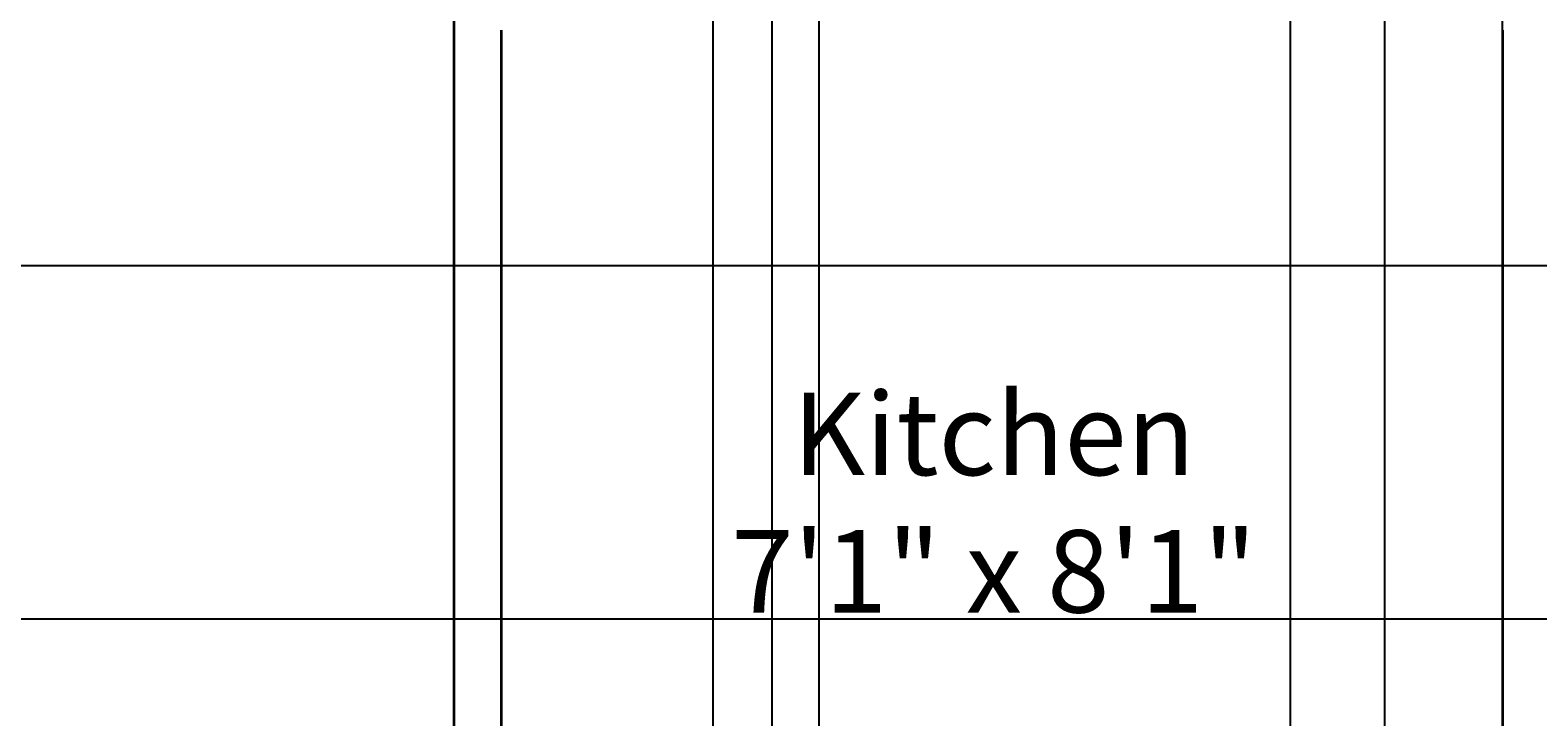
# Model space of a CAD drawing. Units: feet. Extents: x 105 to 1094, y -88 to 588.
# Tile 28 of 59: x 308 to 436, y 433 to 491. Entities that reach past the tile are written whole.
import ezdxf

# ---------------------------------------------------------------- set-up
doc = ezdxf.new("R2010")
doc.units = ezdxf.units.FT
doc.header["$MEASUREMENT"] = 0
for name, color, linetype, lineweight in [('A-ANNO-DIMS', 2, 'Continuous', 18), ('A-AREA-IDEN', 7, 'Continuous', 18), ('A-WALL', 7, 'Continuous', 35)]:
    doc.layers.add(name, color=color, linetype=linetype, lineweight=lineweight)
doc.styles.get("Standard").update_dxf_attribs({"font": 'arial.ttf'})
doc.dimstyles.get("Standard").update_dxf_attribs({"dimtxt": 0.18, "dimasz": 0.18, "dimexe": 0.18, "dimexo": 0.0625, "dimgap": 0.09, "dimtad": 0, "dimtih": 1, "dimtoh": 1, "dimdec": 4, "dimzin": 0, "dimdsep": 46, "dimtxsty": 'Standard', "dimcen": 0.09, "dimadec": 0, "dimazin": 0, "dimtfac": 1, "dimtdec": 4, "dimtofl": 0, "dimtmove": 0, "dimatfit": 3, "dimfxl": 1, "dimtolj": 1, "dimtzin": 0, "dimarcsym": 0})

# ---------------------------------------------------------------- blocks, each defined once
blk = doc.blocks.new('*D21')
at = {"layer": 'A-ANNO-DIMS', "color": 0, "lineweight": -2, "transparency": 16777216}
for p, q in [((849.63, 543.08), (105.46, 543.08)), ((105.64, 542.9), (105.64, 250.26)), ((105.64, -42.74), (105.64, 249.9)), ((849.63, -42.92), (105.46, -42.92))]:
    blk.add_line(p, q, dxfattribs=at)
at = {"layer": 'A-ANNO-DIMS', "color": 0, "transparency": 16777216}
for points in [[(105.61, 542.9), (105.67, 542.9), (105.64, 543.08)], [(105.61, -42.74), (105.67, -42.74), (105.64, -42.92)]]:
    blk.add_solid(points, dxfattribs=at)
at = {"layer": 'Defpoints', "color": 0, "transparency": 16777216}
for p in [(105.64, 543.08), (849.69, 543.08), (849.69, -42.92)]:
    blk.add_point(p, dxfattribs=at)
at = {"layer": 'A-ANNO-DIMS', "color": 0, "transparency": 16777216, "insert": (105.64, 250.08), "char_height": 0.18, "attachment_point": 5}
blk.add_mtext('\\A1;586', dxfattribs=at)
blk = doc.blocks.new('*D32')
at = {"layer": 'A-ANNO-DIMS', "color": 0, "lineweight": -2, "transparency": 16777216}
for p, q in [((646.63, 471.08), (105.46, 471.08)), ((105.64, 470.9), (105.64, 456.26)), ((105.64, 441.26), (105.64, 455.9)), ((646.63, 441.08), (105.46, 441.08))]:
    blk.add_line(p, q, dxfattribs=at)
at = {"layer": 'A-ANNO-DIMS', "color": 0, "transparency": 16777216}
for points in [[(105.61, 470.9), (105.67, 470.9), (105.64, 471.08)], [(105.61, 441.26), (105.67, 441.26), (105.64, 441.08)]]:
    blk.add_solid(points, dxfattribs=at)
at = {"layer": 'Defpoints', "color": 0, "transparency": 16777216}
for p in [(105.64, 471.08), (646.69, 471.08), (646.69, 441.08)]:
    blk.add_point(p, dxfattribs=at)
at = {"layer": 'A-ANNO-DIMS', "color": 0, "transparency": 16777216, "insert": (105.64, 456.08), "char_height": 0.18, "attachment_point": 5}
blk.add_mtext('\\A1;30', dxfattribs=at)
blk = doc.blocks.new('*D39')
at = {"layer": 'A-ANNO-DIMS', "color": 0, "lineweight": -2, "transparency": 16777216}
for p, q in [((294.69, 204.14), (294.69, 588.31)), ((294.87, 588.13), (332.47, 588.13)), ((370.51, 588.13), (332.91, 588.13)), ((370.69, 204.14), (370.69, 588.31))]:
    blk.add_line(p, q, dxfattribs=at)
at = {"layer": 'A-ANNO-DIMS', "color": 0, "transparency": 16777216}
for points in [[(294.87, 588.16), (294.87, 588.1), (294.69, 588.13)], [(370.51, 588.16), (370.51, 588.1), (370.69, 588.13)]]:
    blk.add_solid(points, dxfattribs=at)
at = {"layer": 'Defpoints', "color": 0, "transparency": 16777216}
for p in [(370.69, 588.13), (294.69, 204.08), (370.69, 204.08)]:
    blk.add_point(p, dxfattribs=at)
at = {"layer": 'A-ANNO-DIMS', "color": 0, "transparency": 16777216, "insert": (332.69, 588.13), "char_height": 0.18, "attachment_point": 5}
blk.add_mtext('\\A1;76', dxfattribs=at)
blk = doc.blocks.new('*D52')
at = {"layer": 'A-ANNO-DIMS', "color": 0, "lineweight": -2, "transparency": 16777216}
for p, q in [((414.69, 394.14), (414.69, 588.31)), ((414.87, 588.13), (423.48, 588.13)), ((432.51, 588.13), (423.9, 588.13)), ((432.69, 394.14), (432.69, 588.31))]:
    blk.add_line(p, q, dxfattribs=at)
at = {"layer": 'A-ANNO-DIMS', "color": 0, "transparency": 16777216}
for points in [[(414.87, 588.16), (414.87, 588.1), (414.69, 588.13)], [(432.51, 588.16), (432.51, 588.1), (432.69, 588.13)]]:
    blk.add_solid(points, dxfattribs=at)
at = {"layer": 'Defpoints', "color": 0, "transparency": 16777216}
for p in [(414.69, 588.13), (414.69, 394.08), (432.69, 394.08)]:
    blk.add_point(p, dxfattribs=at)
at = {"layer": 'A-ANNO-DIMS', "color": 0, "transparency": 16777216, "insert": (423.69, 588.13), "char_height": 0.18, "attachment_point": 5}
blk.add_mtext('\\A1;18', dxfattribs=at)
blk = doc.blocks.new('*D53')
at = {"layer": 'A-ANNO-DIMS', "color": 0, "lineweight": -2, "transparency": 16777216}
for p, q in [((365.69, 394.14), (365.69, 588.31)), ((365.87, 588.13), (389.97, 588.13)), ((414.51, 588.13), (390.41, 588.13)), ((414.69, 394.14), (414.69, 588.31))]:
    blk.add_line(p, q, dxfattribs=at)
at = {"layer": 'A-ANNO-DIMS', "color": 0, "transparency": 16777216}
for points in [[(365.87, 588.16), (365.87, 588.1), (365.69, 588.13)], [(414.51, 588.16), (414.51, 588.1), (414.69, 588.13)]]:
    blk.add_solid(points, dxfattribs=at)
at = {"layer": 'Defpoints', "color": 0, "transparency": 16777216}
for p in [(365.69, 588.13), (365.69, 394.08), (414.69, 394.08)]:
    blk.add_point(p, dxfattribs=at)
at = {"layer": 'A-ANNO-DIMS', "color": 0, "transparency": 16777216, "insert": (390.19, 588.13), "char_height": 0.18, "attachment_point": 5}
blk.add_mtext('\\A1;49', dxfattribs=at)
blk = doc.blocks.new('*D56')
at = {"layer": 'A-ANNO-DIMS', "color": 0, "lineweight": -2, "transparency": 16777216}
for p, q in [((374.69, 252.14), (374.69, 588.31)), ((374.87, 588.13), (398.47, 588.13)), ((422.51, 588.13), (398.91, 588.13)), ((422.69, 252.14), (422.69, 588.31))]:
    blk.add_line(p, q, dxfattribs=at)
at = {"layer": 'A-ANNO-DIMS', "color": 0, "transparency": 16777216}
for points in [[(374.87, 588.16), (374.87, 588.1), (374.69, 588.13)], [(422.51, 588.16), (422.51, 588.1), (422.69, 588.13)]]:
    blk.add_solid(points, dxfattribs=at)
at = {"layer": 'Defpoints', "color": 0, "transparency": 16777216}
for p in [(422.69, 588.13), (374.69, 252.08), (422.69, 252.08)]:
    blk.add_point(p, dxfattribs=at)
at = {"layer": 'A-ANNO-DIMS', "color": 0, "transparency": 16777216, "insert": (398.69, 588.13), "char_height": 0.18, "attachment_point": 5}
blk.add_mtext('\\A1;48', dxfattribs=at)

msp = doc.modelspace()

# ---------------------------------------------------------------- linework, layer by layer
at = {"layer": 'A-WALL'}
for p, q in [((343.6883, 507.0812), (343.6883, 390.0812)), ((347.6883, 491.0812), (347.6883, 394.0812)), ((432.6883, 491.0812), (432.6883, 394.0812))]:
    msp.add_line(p, q, dxfattribs=at)

# ---------------------------------------------------------------- texts
at = {"layer": 'A-AREA-IDEN', "insert": (438.6883, 460.3027), "char_height": 7, "attachment_point": 3}
msp.add_mtext_dynamic_manual_height_columns('\\pxqc;Kitchen  \\P7\'1" x 8\'1"', width=98.34246, gutter_width=1, heights=[0], dxfattribs=at)

# ---------------------------------------------------------------- dimensions: what is measured, and where the dimension line sits
at = {"layer": 'A-ANNO-DIMS'}
for base, p1, p2, picture, middle in [((370.6883, 588.1312), (294.6883, 204.0812), (370.6883, 204.0812), '*D39', (332.6883, 588.1312)), ((365.6883, 588.1312), (414.6883, 394.0812), (365.6883, 394.0812), '*D53', (390.1883, 588.1312)), ((422.6883, 588.1312), (374.6883, 252.0812), (422.6883, 252.0812), '*D56', (398.6883, 588.1312)), ((414.6883, 588.1312), (432.6883, 394.0812), (414.6883, 394.0812), '*D52', (423.6883, 588.1312))]:
    dim = msp.add_linear_dim(base=base, p1=p1, p2=p2, dimstyle='Standard', override={"dimdec": 0, "dimlfac": 1, "dimrnd": 0, "dimzin": 0, "dimdsep": 46, "dimlunit": 2}, dxfattribs=at)
    dim.commit()
    dim.dimension.update_dxf_attribs({"geometry": picture, "text_midpoint": middle})
for base, p1, p2, picture, middle in [((105.6383, 543.0812), (849.6883, -42.9188), (849.6883, 543.0812), '*D21', (105.6383, 250.0812)), ((105.6383, 471.0812), (646.6883, 441.0812), (646.6883, 471.0812), '*D32', (105.6383, 456.0812))]:
    dim = msp.add_linear_dim(base=base, p1=p1, p2=p2, angle=90, dimstyle='Standard', override={"dimdec": 0, "dimlfac": 1, "dimrnd": 0, "dimzin": 0, "dimdsep": 46, "dimlunit": 2}, dxfattribs=at)
    dim.commit()
    dim.dimension.update_dxf_attribs({"geometry": picture, "text_midpoint": middle})

doc.saveas('drawing.dxf')
